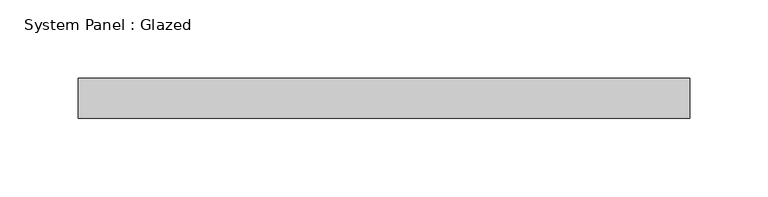
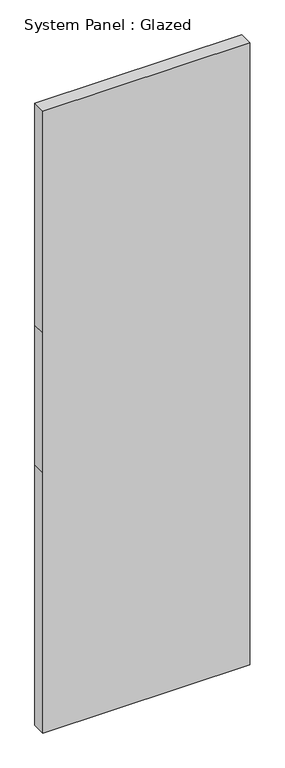
"""IFC4 building model written with IfcOpenShell, lengths in millimetres: plate geometry, System Panel : Glazed."""

from ifc_helpers import new_model, si_unit, frame, origin, place, context, project, spatial, polyline, outline, extrude, source, transform, mapped, element, save


def system_panel_glazed_1b2af392(model_context):
    return source(origin(), model_context, "Body", "SweptSolid", [
        extrude(outline(polyline([(0.0, -195.1407705), (0.0, 195.1407705), (519.0903046, 195.1407705), (797.6854569, 195.1407705), (1239.7709137, 195.1407705), (1239.7709137, -195.1407705), (797.6854569, -195.1407705), (519.0903046, -195.1407705), (0.0, -195.1407705)])), frame((0.0, 19.05, 0.0), z_axis=(0.0, 1.0, 0.0), x_axis=(0.0, 0.0, 1.0)), (0.0, 0.0, 1.0), 25.4),
    ])


if __name__ == "__main__":
    model = new_model("IFC4")
    model_context = context("Model", 3, world=origin())
    ifc_project = project(units=[si_unit("LENGTHUNIT", "METRE", prefix="MILLI")], contexts=[model_context])
    site = spatial("IfcSite", under=ifc_project)
    building = spatial("IfcBuilding", under=site)
    placement = place(None, origin())
    system_panel_glazed_shape = system_panel_glazed_1b2af392(model_context)
    element("IfcPlate", 1, ObjectType="System Panel : Glazed", at=placement, inside=building, context=model_context, shape_type="MappedRepresentation", body=[
        mapped(system_panel_glazed_shape, transform((0.0, 0.0, 0.0), x_axis=(1.0, 0.0, 0.0), y_axis=(0.0, 1.0, 0.0), z_axis=(0.0, 0.0, 1.0))),
    ])
    save(model, "model.ifc")

# Revit data of these elements
# Type "System Panel : Glazed"
#   Construction Type Id = "GSP4R"
#   Analytic Construction = "1/8 in Pilkington single glazing"
#   Visual Light Transmittance = 0.9
#   Solar Heat Gain Coefficient = 0.86
#   Heat Transfer Coefficient (U) = 1.18115 BTU/(h·ft²·°F)
#   Define Thermal Properties by = 1
# Element 1 (IfcPlate, "System Panel : Glazed")
#   Materials on its faces: "Glass"
# Materials
#   "Glass": class "Glass", colour RGB 0 128 192, transparency 0.75, Description = "Soda Lime Glass", Cost = 0
